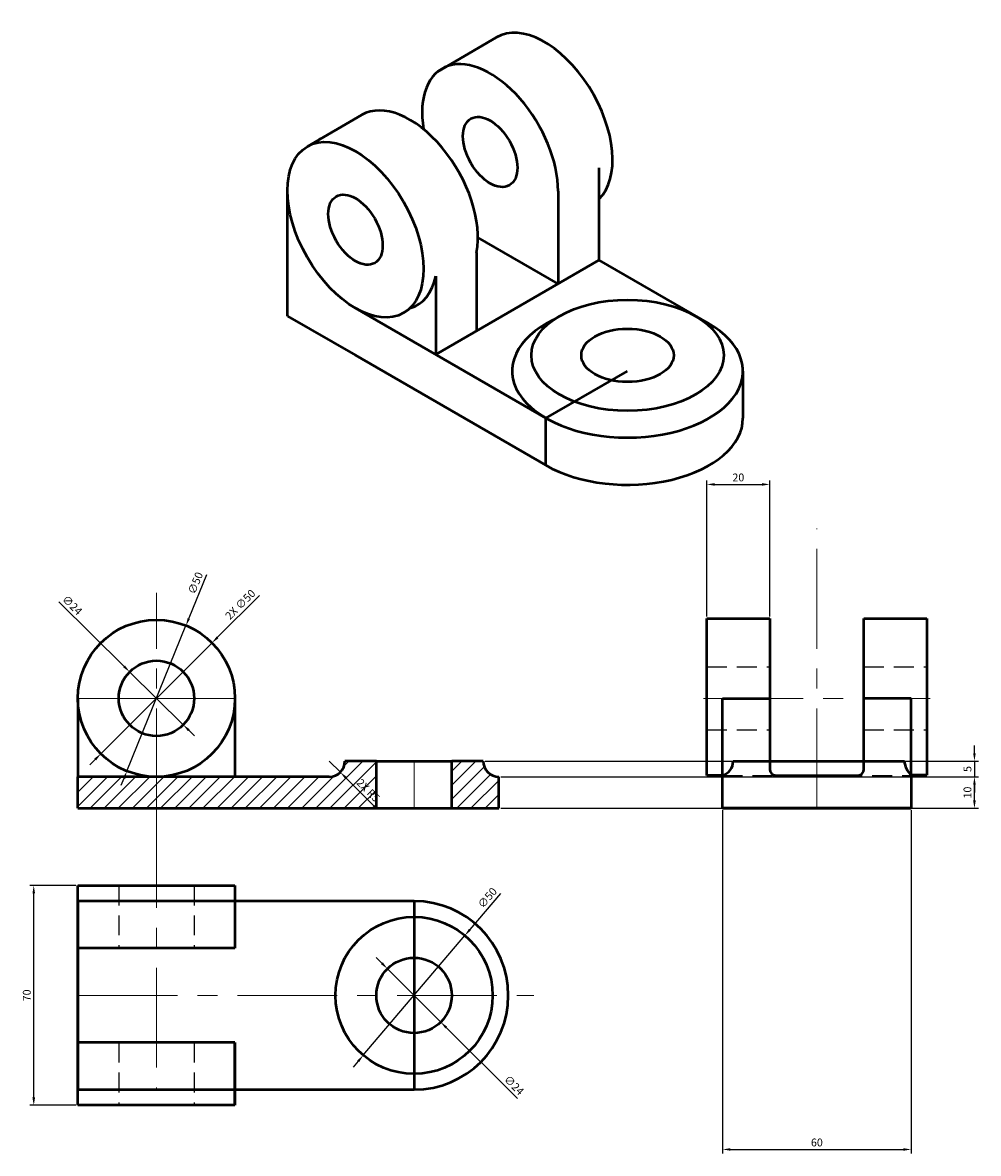
# Model space of a CAD drawing. Units: millimetres. Extents: x 5160 to 5464, y 6001 to 6361.
import ezdxf

# ---------------------------------------------------------------- set-up
doc = ezdxf.new("R2010")
doc.units = ezdxf.units.MM
doc.linetypes.add('CENTER', pattern=[50.8, 31.75, -6.35, 6.35, -6.35])
doc.linetypes.add('HIDDEN', pattern=[9.525, 6.35, -3.175])
for name, color, linetype, lineweight in [('M-CNTR', 1, 'CENTER', 18), ('M-DIMS', 2, 'Continuous', 25), ('M-HATC', 8, 'Continuous', 18), ('M-HIDN', 6, 'HIDDEN', 25), ('M-OUTL', 7, 'Continuous', 50)]:
    doc.layers.add(name, color=color, linetype=linetype, lineweight=lineweight)
doc.styles.get("Standard").update_dxf_attribs({"font": 'arial.ttf'})
doc.dimstyles.new('ISO-25', dxfattribs={"dimtxt": 2.5, "dimasz": 2.5, "dimexe": 1.25, "dimexo": 0.625, "dimtad": 1, "dimtxsty": 'Standard', "dimcen": 2.5, "dimadec": 0, "dimazin": 0, "dimtfac": 1, "dimtmove": 0, "dimatfit": 3, "dimfxl": 1, "dimarcsym": 0})

# ---------------------------------------------------------------- blocks, each defined once
blk = doc.blocks.new('*D1')
at = {"layer": 'Defpoints', "color": 0, "transparency": 16777216}
for p in [(5212.11, 6169.21), (5193.31, 6122.88)]:
    blk.add_point(p, dxfattribs=at)
at = {"layer": 'M-DIMS', "color": 0, "lineweight": -2, "transparency": 16777216}
for p, q in [((5218.67, 6185.38), (5213.05, 6171.53)), ((5193.31, 6122.88), (5212.11, 6169.21)), ((5192.37, 6120.56), (5191.43, 6118.25))]:
    blk.add_line(p, q, dxfattribs=at)
at = {"layer": 'M-DIMS', "color": 0, "transparency": 16777216}
for points in [[(5212.66, 6171.69), (5213.43, 6171.37), (5212.11, 6169.21)], [(5191.99, 6120.72), (5192.76, 6120.41), (5193.31, 6122.88)]]:
    blk.add_solid(points, dxfattribs=at)
at = {"layer": 'M-DIMS', "color": 0, "transparency": 16777216, "insert": (5215.42, 6182.63), "char_height": 2.5, "attachment_point": 5, "rotation": 67.9177}
blk.add_mtext('∅50', dxfattribs=at)
blk = doc.blocks.new('*D2')
at = {"layer": 'Defpoints', "color": 0, "transparency": 16777216}
for p in [(5194.17, 6154.48), (5211.25, 6137.62)]:
    blk.add_point(p, dxfattribs=at)
at = {"layer": 'M-DIMS', "color": 0, "lineweight": -2, "transparency": 16777216}
for p, q in [((5171.62, 6176.74), (5192.39, 6156.23)), ((5211.25, 6137.62), (5194.17, 6154.48)), ((5213.03, 6135.86), (5214.81, 6134.1))]:
    blk.add_line(p, q, dxfattribs=at)
at = {"layer": 'M-DIMS', "color": 0, "transparency": 16777216}
for points in [[(5192.68, 6156.53), (5192.1, 6155.94), (5194.17, 6154.48)], [(5213.32, 6136.16), (5212.74, 6135.56), (5211.25, 6137.62)]]:
    blk.add_solid(points, dxfattribs=at)
at = {"layer": 'M-DIMS', "color": 0, "transparency": 16777216, "insert": (5175.69, 6175.49), "char_height": 2.5, "attachment_point": 5, "rotation": 315.3672}
blk.add_mtext('∅24', dxfattribs=at)
blk = doc.blocks.new('*D3')
at = {"layer": 'Defpoints', "color": 0, "transparency": 16777216}
for p in [(5300.88, 6070.53), (5268.54, 6032.4)]:
    blk.add_point(p, dxfattribs=at)
at = {"layer": 'M-DIMS', "color": 0, "lineweight": -2, "transparency": 16777216}
for p, q in [((5312.24, 6083.92), (5302.5, 6072.44)), ((5268.54, 6032.4), (5300.88, 6070.53)), ((5266.92, 6030.5), (5265.3, 6028.59))]:
    blk.add_line(p, q, dxfattribs=at)
at = {"layer": 'M-DIMS', "color": 0, "transparency": 16777216}
for points in [[(5302.18, 6072.71), (5302.82, 6072.17), (5300.88, 6070.53)], [(5266.6, 6030.77), (5267.24, 6030.23), (5268.54, 6032.4)]]:
    blk.add_solid(points, dxfattribs=at)
at = {"layer": 'M-DIMS', "color": 0, "transparency": 16777216, "insert": (5308.29, 6082.32), "char_height": 2.5, "attachment_point": 5, "rotation": 49.6964}
blk.add_mtext('∅50', dxfattribs=at)
blk = doc.blocks.new('*D4')
at = {"layer": 'Defpoints', "color": 0, "transparency": 16777216}
for p in [(5276.22, 6059.95), (5293.19, 6042.98)]:
    blk.add_point(p, dxfattribs=at)
at = {"layer": 'M-DIMS', "color": 0, "lineweight": -2, "transparency": 16777216}
for p, q in [((5274.46, 6061.72), (5272.69, 6063.49)), ((5276.22, 6059.95), (5293.19, 6042.98)), ((5317.58, 6018.59), (5294.96, 6041.21))]:
    blk.add_line(p, q, dxfattribs=at)
at = {"layer": 'M-DIMS', "color": 0, "transparency": 16777216}
for points in [[(5274.75, 6062.02), (5274.16, 6061.43), (5276.22, 6059.95)], [(5295.26, 6041.51), (5294.67, 6040.92), (5293.19, 6042.98)]]:
    blk.add_solid(points, dxfattribs=at)
at = {"layer": 'M-DIMS', "color": 0, "transparency": 16777216, "insert": (5316.31, 6022.65), "char_height": 2.5, "attachment_point": 5, "rotation": 314.996}
blk.add_mtext('∅24', dxfattribs=at)
blk = doc.blocks.new('*D5')
at = {"layer": 'Defpoints', "color": 0, "transparency": 16777216}
for p in [(5163.66, 6086.47), (5177.71, 6086.47), (5177.71, 6016.47)]:
    blk.add_point(p, dxfattribs=at)
at = {"layer": 'M-DIMS', "color": 0, "lineweight": -2, "transparency": 16777216}
for p, q in [((5177.08, 6086.47), (5162.41, 6086.47)), ((5163.66, 6018.97), (5163.66, 6083.97)), ((5177.08, 6016.47), (5162.41, 6016.47))]:
    blk.add_line(p, q, dxfattribs=at)
at = {"layer": 'M-DIMS', "color": 0, "transparency": 16777216}
for points in [[(5163.24, 6083.97), (5164.08, 6083.97), (5163.66, 6086.47)], [(5163.24, 6018.97), (5164.08, 6018.97), (5163.66, 6016.47)]]:
    blk.add_solid(points, dxfattribs=at)
at = {"layer": 'M-DIMS', "color": 0, "transparency": 16777216, "insert": (5161.76, 6051.47), "char_height": 2.5, "attachment_point": 5, "rotation": 90}
blk.add_mtext('70', dxfattribs=at)
blk = doc.blocks.new('*D6')
at = {"layer": 'Defpoints', "color": 0, "transparency": 16777216}
for p in [(5311.71, 6121.05), (5463.07, 6121.05), (5311.71, 6111.05)]:
    blk.add_point(p, dxfattribs=at)
at = {"layer": 'M-DIMS', "color": 0, "lineweight": -2, "transparency": 16777216}
for p, q in [((5312.33, 6121.05), (5464.32, 6121.05)), ((5463.07, 6113.55), (5463.07, 6118.55)), ((5312.33, 6111.05), (5464.32, 6111.05))]:
    blk.add_line(p, q, dxfattribs=at)
at = {"layer": 'M-DIMS', "color": 0, "transparency": 16777216}
for points in [[(5462.66, 6118.55), (5463.49, 6118.55), (5463.07, 6121.05)], [(5462.66, 6113.55), (5463.49, 6113.55), (5463.07, 6111.05)]]:
    blk.add_solid(points, dxfattribs=at)
at = {"layer": 'M-DIMS', "color": 0, "transparency": 16777216, "insert": (5461.17, 6116.05), "char_height": 2.5, "attachment_point": 5, "rotation": 90}
blk.add_mtext('10', dxfattribs=at)
blk = doc.blocks.new('*D7')
at = {"layer": 'Defpoints', "color": 0, "transparency": 16777216}
for p in [(5306.71, 6126.05), (5311.71, 6121.05), (5463.07, 6121.05)]:
    blk.add_point(p, dxfattribs=at)
at = {"layer": 'M-DIMS', "color": 0, "lineweight": -2, "transparency": 16777216}
for p, q in [((5463.07, 6128.55), (5463.07, 6131.05)), ((5307.33, 6126.05), (5464.32, 6126.05)), ((5463.07, 6126.05), (5463.07, 6121.05)), ((5312.33, 6121.05), (5464.32, 6121.05)), ((5463.07, 6118.55), (5463.07, 6116.05))]:
    blk.add_line(p, q, dxfattribs=at)
at = {"layer": 'M-DIMS', "color": 0, "transparency": 16777216}
for points in [[(5462.66, 6128.55), (5463.49, 6128.55), (5463.07, 6126.05)], [(5462.66, 6118.55), (5463.49, 6118.55), (5463.07, 6121.05)]]:
    blk.add_solid(points, dxfattribs=at)
at = {"layer": 'M-DIMS', "color": 0, "transparency": 16777216, "insert": (5461.18, 6123.55), "char_height": 2.5, "attachment_point": 5, "rotation": 90}
blk.add_mtext('5', dxfattribs=at)
blk = doc.blocks.new('*D8')
at = {"layer": 'Defpoints', "color": 0, "transparency": 16777216}
for p in [(5397.92, 6214.15), (5377.92, 6171.5), (5397.92, 6171.5)]:
    blk.add_point(p, dxfattribs=at)
at = {"layer": 'M-DIMS', "color": 0, "lineweight": -2, "transparency": 16777216}
for p, q in [((5377.92, 6172.12), (5377.92, 6215.4)), ((5380.42, 6214.15), (5395.42, 6214.15)), ((5397.92, 6172.12), (5397.92, 6215.4))]:
    blk.add_line(p, q, dxfattribs=at)
at = {"layer": 'M-DIMS', "color": 0, "transparency": 16777216}
for points in [[(5380.42, 6214.57), (5380.42, 6213.73), (5377.92, 6214.15)], [(5395.42, 6214.57), (5395.42, 6213.73), (5397.92, 6214.15)]]:
    blk.add_solid(points, dxfattribs=at)
at = {"layer": 'M-DIMS', "color": 0, "transparency": 16777216, "insert": (5387.92, 6216.05), "char_height": 2.5, "attachment_point": 5}
blk.add_mtext('20', dxfattribs=at)
blk = doc.blocks.new('*D9')
at = {"layer": 'Defpoints', "color": 0, "transparency": 16777216}
for p in [(5382.92, 6111.05), (5442.92, 6111.05), (5442.92, 6002.42)]:
    blk.add_point(p, dxfattribs=at)
at = {"layer": 'M-DIMS', "color": 0, "lineweight": -2, "transparency": 16777216}
for p, q in [((5382.92, 6110.42), (5382.92, 6001.17)), ((5442.92, 6110.42), (5442.92, 6001.17)), ((5385.42, 6002.42), (5440.42, 6002.42))]:
    blk.add_line(p, q, dxfattribs=at)
at = {"layer": 'M-DIMS', "color": 0, "transparency": 16777216}
for points in [[(5385.42, 6002.83), (5385.42, 6002), (5382.92, 6002.42)], [(5440.42, 6002.83), (5440.42, 6002), (5442.92, 6002.42)]]:
    blk.add_solid(points, dxfattribs=at)
at = {"layer": 'M-DIMS', "color": 0, "transparency": 16777216, "insert": (5412.92, 6004.32), "char_height": 2.5, "attachment_point": 5}
blk.add_mtext('60', dxfattribs=at)
blk = doc.blocks.new('*D10')
at = {"layer": 'Defpoints', "color": 0, "transparency": 16777216}
for p in [(5257.71, 6126.05), (5261.25, 6122.51)]:
    blk.add_point(p, dxfattribs=at)
at = {"layer": 'M-DIMS', "color": 0, "lineweight": -2, "transparency": 16777216}
for p, q in [((5257.71, 6126.05), (5261.25, 6122.51)), ((5272.36, 6111.4), (5263.01, 6120.74))]:
    blk.add_line(p, q, dxfattribs=at)
at = {"layer": 'M-DIMS', "color": 0, "transparency": 16777216}
blk.add_solid([(5263.31, 6121.04), (5262.72, 6120.45), (5261.25, 6122.51)], dxfattribs=at)
at = {"layer": 'M-DIMS', "color": 0, "transparency": 16777216, "insert": (5269.91, 6116.53), "char_height": 2.5, "attachment_point": 5, "rotation": 315.0021}
blk.add_mtext('2X R5', dxfattribs=at)
blk = doc.blocks.new('*D11')
at = {"layer": 'Defpoints', "color": 0, "transparency": 16777216}
for p in [(5220.41, 6163.71), (5185.01, 6128.39)]:
    blk.add_point(p, dxfattribs=at)
at = {"layer": 'M-DIMS', "color": 0, "lineweight": -2, "transparency": 16777216}
for p, q in [((5235.56, 6178.83), (5222.18, 6165.47)), ((5185.01, 6128.39), (5220.41, 6163.71)), ((5183.24, 6126.62), (5181.47, 6124.86))]:
    blk.add_line(p, q, dxfattribs=at)
at = {"layer": 'M-DIMS', "color": 0, "transparency": 16777216}
for points in [[(5221.88, 6165.77), (5222.47, 6165.18), (5220.41, 6163.71)], [(5182.95, 6126.92), (5183.54, 6126.33), (5185.01, 6128.39)]]:
    blk.add_solid(points, dxfattribs=at)
at = {"layer": 'M-DIMS', "color": 0, "transparency": 16777216, "insert": (5229.63, 6175.7), "char_height": 2.5, "attachment_point": 5, "rotation": 44.9403}
blk.add_mtext('2X ∅50', dxfattribs=at)

msp = doc.modelspace()

# ---------------------------------------------------------------- hatches: boundary and pattern name
at = {"layer": 'M-HATC'}
h = msp.add_hatch(dxfattribs=at)
h.set_pattern_fill('ANSI31', color=256)
h.paths.add_polyline_path([(5202.709, 6121.046), (5177.709, 6121.046), (5177.709, 6111.046), (5202.709, 6111.046)])
h.paths.add_polyline_path([(5272.709, 6126.046), (5262.709, 6126.046, -0.4142136), (5257.709, 6121.046), (5202.709, 6121.046), (5202.709, 6111.046), (5272.709, 6111.046)])
h.paths.add_polyline_path([(5311.709, 6121.046, -0.4142136), (5306.709, 6126.046), (5296.709, 6126.046), (5296.709, 6111.046), (5311.709, 6111.046)])

# ---------------------------------------------------------------- linework, layer by layer
at = {"layer": 'M-CNTR'}
for p, q in [((5412.916, 6111.046), (5412.916, 6200.101)), ((5202.709, 6111.046), (5202.709, 6179.587)), ((5202.709, 6146.046), (5177.709, 6146.046)), ((5202.709, 6146.046), (5214.709, 6146.046)), ((5214.709, 6146.046), (5227.709, 6146.046)), ((5376.807, 6146.046), (5449.024, 6146.046)), ((5377.916, 6146.046), (5397.916, 6146.046)), ((5427.916, 6146.046), (5447.916, 6146.046)), ((5284.709, 6111.046), (5284.709, 6126.046)), ((5202.709, 6111.046), (5202.709, 6021.468)), ((5177.709, 6051.468), (5322.817, 6051.468))]:
    msp.add_line(p, q, dxfattribs=at)
at = {"layer": 'M-HIDN'}
for p, q in [((5377.916, 6156.046), (5397.916, 6156.046)), ((5427.916, 6156.046), (5447.916, 6156.046)), ((5377.916, 6136.046), (5397.916, 6136.046)), ((5427.916, 6136.046), (5447.916, 6136.046)), ((5382.916, 6121.497), (5442.916, 6121.497)), ((5190.709, 6086.468), (5190.709, 6066.468)), ((5214.709, 6086.468), (5214.709, 6066.468)), ((5190.709, 6036.468), (5190.709, 6016.468)), ((5214.709, 6036.468), (5214.709, 6016.468))]:
    msp.add_line(p, q, dxfattribs=at)
at = {"layer": 'M-OUTL'}
for p, q in [((5292.16, 6345.506), (5310.868, 6356.483)), ((5250.746, 6321.771), (5268.066, 6331.771)), ((5343.56, 6315.002), (5343.56, 6285.507)), ((5244.404, 6267.755), (5244.404, 6307.755)), ((5330.569, 6307.502), (5330.569, 6278.007)), ((5330.569, 6278.007), (5305.026, 6292.755)), ((5304.589, 6288.007), (5304.589, 6263.007)), ((5291.598, 6255.507), (5343.56, 6285.507)), ((5343.56, 6285.507), (5378.638, 6265.255)), ((5291.598, 6280.507), (5291.598, 6255.507)), ((5326.677, 6235.255), (5266.055, 6270.255)), ((5244.404, 6267.755), (5266.055, 6255.255)), ((5266.055, 6255.255), (5326.677, 6220.255)), ((5326.677, 6235.255), (5352.657, 6250.255)), ((5389.4, 6250.255), (5389.4, 6235.255)), ((5326.677, 6220.255), (5326.677, 6235.255)), ((5377.916, 6121.497), (5377.916, 6171.497)), ((5377.916, 6171.497), (5397.916, 6171.497)), ((5397.916, 6171.497), (5397.916, 6123.497)), ((5427.916, 6123.497), (5427.916, 6171.497)), ((5427.916, 6171.497), (5447.916, 6171.497)), ((5447.916, 6171.497), (5447.916, 6121.594)), ((5177.709, 6146.046), (5177.709, 6121.046)), ((5227.709, 6146.046), (5227.709, 6121.046)), ((5382.916, 6121.497), (5382.916, 6146.046)), ((5382.916, 6146.046), (5397.916, 6146.046)), ((5442.916, 6146.046), (5427.916, 6146.046)), ((5442.916, 6121.594), (5442.916, 6146.046)), ((5272.709, 6126.046), (5262.709, 6126.046)), ((5262.709, 6126.046), (5262.709, 6126.046)), ((5272.709, 6111.046), (5272.709, 6126.046)), ((5272.709, 6126.046), (5296.709, 6126.046)), ((5296.709, 6111.046), (5296.709, 6126.046)), ((5306.709, 6126.046), (5296.709, 6126.046)), ((5306.709, 6126.046), (5296.709, 6126.046)), ((5306.709, 6126.046), (5306.709, 6126.046)), ((5386.253, 6126.046), (5440.778, 6126.046)), ((5257.709, 6121.046), (5177.709, 6121.046)), ((5177.709, 6111.046), (5177.709, 6121.046)), ((5311.709, 6111.046), (5311.709, 6121.046)), ((5311.709, 6121.046), (5311.709, 6121.046)), ((5382.916, 6121.497), (5377.916, 6121.497)), ((5382.916, 6111.046), (5382.916, 6121.497)), ((5399.916, 6121.497), (5425.916, 6121.497)), ((5442.916, 6121.594), (5442.916, 6111.046)), ((5447.916, 6121.594), (5442.916, 6121.594)), ((5177.709, 6111.046), (5202.709, 6111.046)), ((5202.709, 6111.046), (5272.709, 6111.046)), ((5272.709, 6111.046), (5296.709, 6111.046)), ((5296.709, 6111.046), (5311.709, 6111.046)), ((5382.916, 6111.046), (5442.916, 6111.046)), ((5442.916, 6111.046), (5382.916, 6111.046)), ((5177.709, 6021.468), (5177.709, 6086.468)), ((5177.709, 6086.468), (5227.709, 6086.468)), ((5227.709, 6086.468), (5227.709, 6066.468)), ((5227.709, 6086.468), (5227.709, 6066.468)), ((5177.709, 6081.468), (5177.709, 6021.468)), ((5284.709, 6081.468), (5177.709, 6081.468)), ((5284.709, 6081.468), (5284.709, 6021.468)), ((5227.709, 6066.468), (5177.709, 6066.468)), ((5227.709, 6036.468), (5177.709, 6036.468)), ((5227.709, 6016.468), (5227.709, 6036.468)), ((5227.709, 6036.468), (5227.709, 6016.468)), ((5177.709, 6021.468), (5284.709, 6021.468)), ((5177.709, 6016.468), (5177.709, 6021.468)), ((5227.709, 6016.468), (5177.709, 6016.468))]:
    msp.add_line(p, q, dxfattribs=at)
for centre, radius in [((5202.709, 6146.046), 25), ((5202.709, 6146.046), 12), ((5284.709, 6051.468), 25), ((5284.709, 6051.468), 12)]:
    msp.add_circle(centre, radius, dxfattribs=at)
for centre, radius, start, end in [((5257.709, 6126.046), 5, 270, 0), ((5311.709, 6126.046), 5, 180, 270), ((5381.484, 6126.046), 4.77, 287.47341, 0), ((5447.193, 6126.386), 6.423, 183.03448, 228.25398), ((5399.916, 6123.497), 2, 180, 270), ((5425.916, 6123.497), 2, 270, 0), ((5284.709, 6051.468), 30, 270, 90)]:
    msp.add_arc(centre, radius, start, end, dxfattribs=at)
for centre, major_axis, start_param, end_param in [((5326.239, 6330.002), (15.309, -26.517), 6.4250824, 9.428829), ((5308.919, 6320.002), (15.309, -26.517), 7.0685835, 10.411534), ((5283.375, 6305.255), (15.309, -26.517), 0.5840402, 3.1415927), ((5270.385, 6297.755), (15.309, -26.517), 3.1415927, 3.2834897), ((5270.385, 6297.755), (15.309, -26.517), 6.1412883, 6.8672255), ((5352.657, 6250.255), (-36.742, 0), 5.4105395, 10.2974238), ((5352.657, 6235.255), (-36.742, 0), 7.0685835, 9.424778)]:
    msp.add_ellipse(centre, major_axis=major_axis, ratio=0.5773503, start_param=start_param, end_param=end_param, dxfattribs=at)
for centre, major_axis in [((5308.919, 6320.002), (6.124, -10.607)), ((5266.055, 6295.255), (15.309, -26.517)), ((5266.055, 6295.255), (6.124, -10.607)), ((5352.657, 6255.255), (-30.619, 0)), ((5352.657, 6255.255), (-14.697, 0))]:
    msp.add_ellipse(centre, major_axis=major_axis, ratio=0.5773503, dxfattribs=at)

# ---------------------------------------------------------------- dimensions: what is measured, and where the dimension line sits
at = {"layer": 'M-DIMS'}
for base, p1, p2, picture, middle in [((5397.916, 6214.151), (5377.916, 6171.497), (5397.916, 6171.497), '*D8', (5387.916, 6216.053)), ((5442.916, 6002.418), (5382.916, 6111.046), (5442.916, 6111.046), '*D9', (5412.916, 6004.319))]:
    dim = msp.add_linear_dim(base=base, p1=p1, p2=p2, dimstyle='ISO-25', override={"dimdec": 0, "dimlfac": 1, "dimrnd": 0, "dimzin": 0, "dimdsep": 46, "dimlunit": 2}, dxfattribs=at)
    dim.commit()
    dim.dimension.update_dxf_attribs({"geometry": picture, "text_midpoint": middle})
for p1, p2, picture, middle in [((5193.311, 6122.88), (5212.108, 6169.212), '*D1', (5217.249, 6181.884)), ((5211.249, 6137.616), (5194.17, 6154.477), '*D2', (5174.304, 6174.09)), ((5268.539, 6032.402), (5300.88, 6070.533), '*D3', (5309.798, 6081.047)), ((5276.225, 6059.954), (5293.194, 6042.982), '*D4', (5314.919, 6021.254))]:
    dim = msp.add_diameter_dim_2p(p1=p1, p2=p2, dimstyle='ISO-25', override={"dimclrd": 0, "dimclre": 0, "dimclrt": 0}, dxfattribs=at)
    dim.commit()
    dim.dimension.update_dxf_attribs({"geometry": picture, "text_midpoint": middle, "dimtype": 163})
dim = msp.add_diameter_dim_2p(p1=(5185.013, 6128.387), p2=(5220.406, 6163.706), text='2X <>', dimstyle='ISO-25', override={"dimdec": 0, "dimlfac": 1, "dimrnd": 0, "dimzin": 0, "dimdsep": 46, "dimlunit": 2}, dxfattribs=at)
dim.commit()
dim.dimension.update_dxf_attribs({"geometry": '*D11', "text_midpoint": (5231.023, 6174.301), "dimtype": 163})
for base, p1, p2, picture, middle in [((5463.074, 6121.046), (5306.709, 6126.046), (5311.709, 6121.046), '*D7', (5461.178, 6123.546)), ((5463.074, 6121.046), (5311.709, 6111.046), (5311.709, 6121.046), '*D6', (5461.173, 6116.046)), ((5163.659, 6086.468), (5177.709, 6016.468), (5177.709, 6086.468), '*D5', (5161.758, 6051.468))]:
    dim = msp.add_linear_dim(base=base, p1=p1, p2=p2, angle=90, dimstyle='ISO-25', override={"dimdec": 0, "dimlfac": 1, "dimrnd": 0, "dimzin": 0, "dimdsep": 46, "dimlunit": 2}, dxfattribs=at)
    dim.commit()
    dim.dimension.update_dxf_attribs({"geometry": picture, "text_midpoint": middle})
dim = msp.add_radius_dim(center=(5257.709, 6126.046), mpoint=(5261.245, 6122.511), text='2X <>', dimstyle='ISO-25', override={"dimdec": 0, "dimlfac": 1, "dimrnd": 0, "dimzin": 0, "dimdsep": 46, "dimlunit": 2}, dxfattribs=at)
dim.commit()
dim.dimension.update_dxf_attribs({"geometry": '*D10', "text_midpoint": (5269.914, 6116.532)})

doc.saveas('drawing.dxf')
